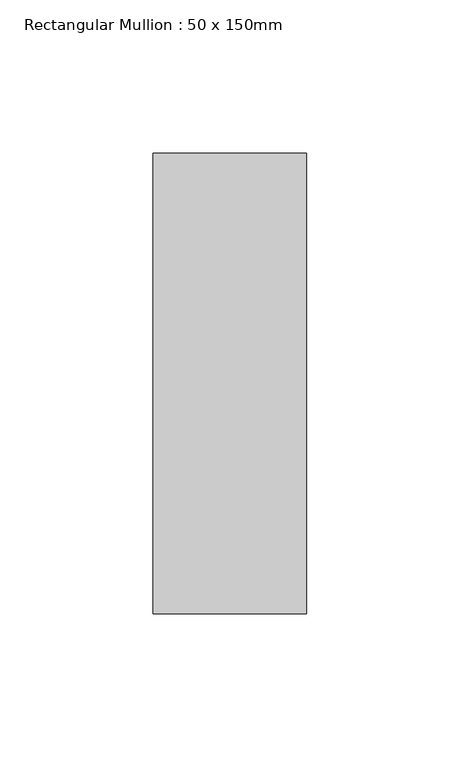
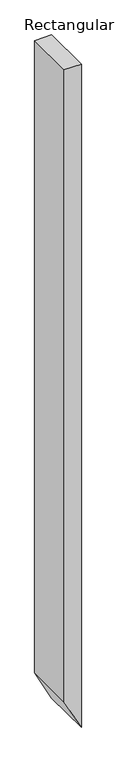
"""IFC4 building model written with IfcOpenShell, lengths in millimetres: member geometry, Rectangular Mullion : 50 x 150mm."""

from ifc_helpers import new_model, si_unit, frame, origin, place, context, project, spatial, polyline, outline, extrude, source, transform, mapped, element, save


def rectangular_mullion_50_x_150mm_b2f97b5b(model_context):
    return source(origin(), model_context, "Body", "SweptSolid", [
        extrude(outline(polyline([(0.0, 0.0), (0.0, -50.0), (-1956.0404197, -50.0), (-2052.089526, 0.0), (0.0, 0.0)])), frame((0.0, -75.0, 0.0), z_axis=(0.0, 1.0, 0.0), x_axis=(0.0, 0.0, 1.0)), (0.0, 0.0, 1.0), 150.0),
    ])


if __name__ == "__main__":
    model = new_model("IFC4")
    model_context = context("Model", 3, world=origin())
    ifc_project = project(units=[si_unit("LENGTHUNIT", "METRE", prefix="MILLI")], contexts=[model_context])
    site = spatial("IfcSite", under=ifc_project)
    building = spatial("IfcBuilding", under=site)
    placement = place(None, origin())
    rectangular_mullion_50_x_150mm_shape = rectangular_mullion_50_x_150mm_b2f97b5b(model_context)
    element("IfcMember", 1, ObjectType="Rectangular Mullion : 50 x 150mm", at=placement, inside=building, context=model_context, shape_type="MappedRepresentation", body=[
        mapped(rectangular_mullion_50_x_150mm_shape, transform((0.0, 0.0, 0.0), x_axis=(1.0, 0.0, 0.0), y_axis=(0.0, 1.0, 0.0), z_axis=(0.0, 0.0, 1.0))),
    ])
    save(model, "model.ifc")

# Revit data of these elements
# Type "Rectangular Mullion : 50 x 150mm"
#   built-in parameter 1007304 = 0.492126 (stored number, unit not read)
#   built-in parameter 1007301 = 0.082021 (stored number, unit not read)
#   built-in parameter 1007300 = 0.082021 (stored number, unit not read)
# Element 1 (IfcMember, "Rectangular Mullion : 50 x 150mm")
#   Materials on its faces: "Aluminium"
# Materials
#   "Aluminium": class "Metal", colour RGB 247 247 247, transparency 0, Description = "Aluminium 6061", Cost = 0
